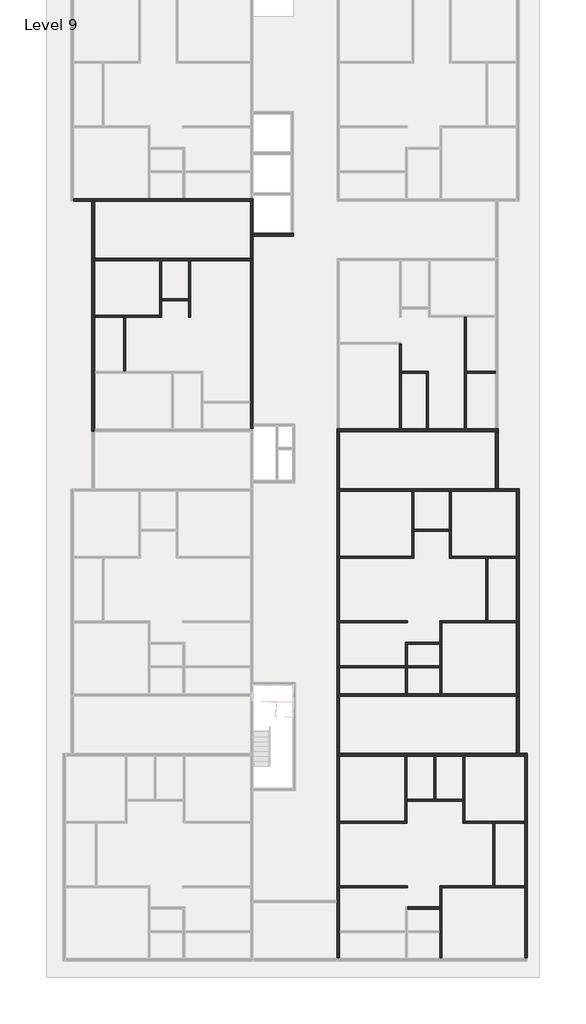
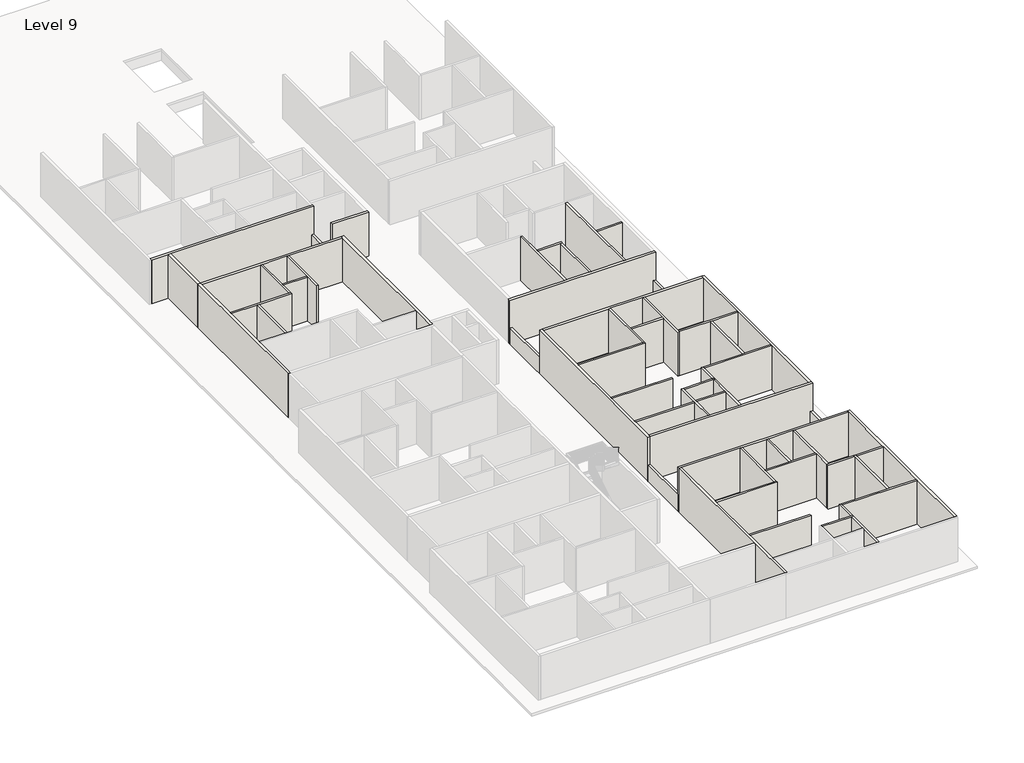
# One storey, part 2 of 8: 56 walls.
"""IFC4 building model written with IfcOpenShell, lengths in millimetres."""

from ifc_helpers import new_model, si_unit, frame, origin, place, context, project, spatial, polyline, outline, extrude, faceted_brep, element, save

model = new_model("IFC4")

# Units and contexts
model_context = context("Model", 3, world=origin())
ifc_project = project(units=[si_unit("LENGTHUNIT", "METRE", prefix="MILLI")], contexts=[model_context])

# Site, building, storey
site = spatial("IfcSite", under=ifc_project)
building = spatial("IfcBuilding", under=site)
storey = spatial("IfcBuildingStorey", under=building, Name="Level 9", Elevation=49618.6172466)

# Walls
placement = place(None, origin())
element("IfcWall", 1, ObjectType="4.5\"", at=placement, inside=storey, context=model_context, shape_type="Brep", body=[
    faceted_brep([(-12531.5544854, 2100.0216096, 49618.6172466), (-10907.2415084, 2100.0216096, 49618.6172466), (-10792.9415084, 2100.0216096, 49618.6172466), (-8759.6544854, 2100.0216096, 49618.6172466), (-8759.6544854, 2100.0216096, 52666.6172466), (-10792.9415084, 2100.0216096, 52666.6172466), (-10907.2415084, 2100.0216096, 52666.6172466), (-12531.5544854, 2100.0216096, 52666.6172466), (-12531.5544854, 2214.3216096, 49618.6172466), (-12531.5544854, 2214.3216096, 52666.6172466), (-8873.9544854, 2214.3216096, 52666.6172466), (-8759.6544854, 2214.3216096, 52666.6172466), (-8759.6544854, 2214.3216096, 49618.6172466), (-8873.9544854, 2214.3216096, 49618.6172466)], [[[0, 1, 2, 3, 4, 5, 6, 7]], [[8, 9, 10, 11, 12, 13]], [[3, 2, 1, 0, 8, 13, 12]], [[0, 7, 9, 8]], [[4, 3, 12, 11]], [[7, 6, 5, 4, 11, 10, 9]]]),
])
element("IfcWall", 2, ObjectType="4.5\"", at=placement, inside=storey, context=model_context, shape_type="Brep", body=[
    faceted_brep([(-8759.6544854, 2214.3216096, 49618.6172466), (-8759.6544854, 3014.4216096, 49618.6172466), (-8759.6544854, 3128.7216096, 49618.6172466), (-8759.6544854, 5264.2743917, 49618.6172466), (-8759.6544854, 5264.2743917, 52666.6172466), (-8759.6544854, 3128.7216096, 52666.6172466), (-8759.6544854, 3014.4216096, 52666.6172466), (-8759.6544854, 2214.3216096, 52666.6172466), (-8873.9544854, 2214.3216096, 49618.6172466), (-8873.9544854, 2214.3216096, 52666.6172466), (-8873.9544854, 5264.2743917, 52666.6172466), (-8873.9544854, 5264.2743917, 49618.6172466)], [[[0, 1, 2, 3, 4, 5, 6, 7]], [[8, 9, 10, 11]], [[3, 2, 1, 0, 8, 11]], [[0, 7, 9, 8]], [[4, 3, 11, 10]], [[7, 6, 5, 4, 10, 9]]]),
])
element("IfcWall", 3, ObjectType="4.5\"", at=placement, inside=storey, context=model_context, shape_type="Brep", body=[
    faceted_brep([(-7235.6544854, 5264.2743917, 49618.6172466), (-7235.6544854, 3128.7216096, 49618.6172466), (-7235.6544854, 3014.4216096, 49618.6172466), (-7235.6544854, 2100.0216096, 49618.6172466), (-7235.6544854, 2100.0216096, 52666.6172466), (-7235.6544854, 3014.4216096, 52666.6172466), (-7235.6544854, 3128.7216096, 52666.6172466), (-7235.6544854, 5264.2743917, 52666.6172466), (-7121.3544854, 5264.2743917, 49618.6172466), (-7121.3544854, 5264.2743917, 52666.6172466), (-7121.3544854, 2100.0216096, 52666.6172466), (-7121.3544854, 2100.0216096, 49618.6172466)], [[[0, 1, 2, 3, 4, 5, 6, 7]], [[8, 9, 10, 11]], [[3, 2, 1, 0, 8, 11]], [[4, 3, 11, 10]], [[0, 7, 9, 8]], [[7, 6, 5, 4, 10, 9]]]),
])
element("IfcWall", 4, ObjectType="4.5\"", at=placement, inside=storey, context=model_context, shape_type="SweptSolid", body=[
    extrude(outline(polyline([(-7235.6544854, 3014.4216096), (-8759.6544854, 3014.4216096), (-8759.6544854, 3128.7216096), (-7235.6544854, 3128.7216096), (-7235.6544854, 3014.4216096)])), frame((0.0, 0.0, 49618.6172466), z_axis=(0.0, 0.0, 1.0), x_axis=(1.0, 0.0, 0.0)), (0.0, 0.0, 1.0), 3048.0),
])
element("IfcWall", 5, ObjectType="4.5\"", at=placement, inside=storey, context=model_context, shape_type="SweptSolid", body=[
    extrude(outline(polyline([(-10907.2415084, -947.4344126), (-10907.2415084, 2100.0216096), (-10792.9415084, 2100.0216096), (-10792.9415084, -947.4344126), (-10907.2415084, -947.4344126)])), frame((0.0, 0.0, 49618.6172466), z_axis=(0.0, 0.0, 1.0), x_axis=(1.0, 0.0, 0.0)), (0.0, 0.0, 1.0), 3048.0),
])
element("IfcWall", 6, ObjectType="4.5\"", at=placement, inside=storey, context=model_context, shape_type="Brep", body=[
    faceted_brep([(5056.6584916, -31173.4344126, 49618.6172466), (6885.4584916, -31173.4344126, 49618.6172466), (6999.7584916, -31173.4344126, 49618.6172466), (6999.7584916, -31173.4344126, 52666.6172466), (6885.4584916, -31173.4344126, 52666.6172466), (5056.6584916, -31173.4344126, 52666.6172466), (5056.6584916, -31059.1344126, 49618.6172466), (5056.6584916, -31059.1344126, 52666.6172466), (6885.4584916, -31059.1344126, 52666.6172466), (6999.7584916, -31059.1344126, 52666.6172466), (6999.7584916, -31059.1344126, 49618.6172466), (6885.4584916, -31059.1344126, 49618.6172466)], [[[0, 1, 2, 3, 4, 5]], [[6, 7, 8, 9, 10, 11]], [[2, 1, 0, 6, 11, 10]], [[0, 5, 7, 6]], [[3, 2, 10, 9]], [[5, 4, 3, 9, 8, 7]]]),
])
element("IfcWall", 7, ObjectType="4.5\"", at=placement, inside=storey, context=model_context, shape_type="Brep", body=[
    faceted_brep([(6885.4584916, -31173.4344126, 49618.6172466), (6885.4584916, -32392.6344126, 49618.6172466), (6885.4584916, -32506.9344126, 49618.6172466), (6885.4584916, -33954.7344126, 49618.6172466), (6885.4584916, -33954.7344126, 52666.6172466), (6885.4584916, -32506.9344126, 52666.6172466), (6885.4584916, -32392.6344126, 52666.6172466), (6885.4584916, -31173.4344126, 52666.6172466), (6999.7584916, -31173.4344126, 49618.6172466), (6999.7584916, -31173.4344126, 52666.6172466), (6999.7584916, -33954.7344126, 52666.6172466), (6999.7584916, -33954.7344126, 49618.6172466)], [[[0, 1, 2, 3, 4, 5, 6, 7]], [[8, 9, 10, 11]], [[3, 2, 1, 0, 8, 11]], [[0, 7, 9, 8]], [[4, 3, 11, 10]], [[7, 6, 5, 4, 10, 9]]]),
])
element("IfcWall", 8, ObjectType="4.5\"", at=placement, inside=storey, context=model_context, shape_type="Brep", body=[
    faceted_brep([(6999.7584916, -31059.1344126, 49618.6172466), (6999.7584916, -29966.9344126, 49618.6172466), (6999.7584916, -29852.6344126, 49618.6172466), (6999.7584916, -29852.6344126, 52666.6172466), (6999.7584916, -29966.9344126, 52666.6172466), (6999.7584916, -31059.1344126, 52666.6172466), (6885.4584916, -31059.1344126, 49618.6172466), (6885.4584916, -31059.1344126, 52666.6172466), (6885.4584916, -29852.6344126, 52666.6172466), (6885.4584916, -29852.6344126, 49618.6172466)], [[[0, 1, 2, 3, 4, 5]], [[6, 7, 8, 9]], [[2, 1, 0, 6, 9]], [[0, 5, 7, 6]], [[3, 2, 9, 8]], [[5, 4, 3, 8, 7]]]),
])
element("IfcWall", 9, ObjectType="4.5\"", at=placement, inside=storey, context=model_context, shape_type="Brep", body=[
    faceted_brep([(6999.7584916, -29966.9344126, 49618.6172466), (11660.6584916, -29966.9344126, 49618.6172466), (11660.6584916, -29966.9344126, 52666.6172466), (6999.7584916, -29966.9344126, 52666.6172466), (6999.7584916, -29852.6344126, 49618.6172466), (6999.7584916, -29852.6344126, 52666.6172466), (9869.9584916, -29852.6344126, 52666.6172466), (9984.2584916, -29852.6344126, 52666.6172466), (11660.6584916, -29852.6344126, 52666.6172466), (11660.6584916, -29852.6344126, 49618.6172466), (9984.2584916, -29852.6344126, 49618.6172466), (9869.9584916, -29852.6344126, 49618.6172466)], [[[0, 1, 2, 3]], [[4, 5, 6, 7, 8, 9, 10, 11]], [[1, 0, 4, 11, 10, 9]], [[0, 3, 5, 4]], [[2, 1, 9, 8]], [[3, 2, 8, 7, 6, 5]]]),
])
element("IfcWall", 10, ObjectType="4.5\"", at=placement, inside=storey, context=model_context, shape_type="SweptSolid", body=[
    extrude(outline(polyline([(5056.6584916, -29966.9344126), (1259.3584916, -29966.9344126), (1259.3584916, -29852.6344126), (5056.6584916, -29852.6344126), (5056.6584916, -29966.9344126)])), frame((0.0, 0.0, 49618.6172466), z_axis=(0.0, 0.0, 1.0), x_axis=(1.0, 0.0, 0.0)), (0.0, 0.0, 1.0), 3048.0),
])
element("IfcWall", 11, ObjectType="4.5\"", at=placement, inside=storey, context=model_context, shape_type="Brep", body=[
    faceted_brep([(1259.3584916, -26347.4344126, 49618.6172466), (5031.2584916, -26347.4344126, 49618.6172466), (5031.2584916, -26347.4344126, 52666.6172466), (1259.3584916, -26347.4344126, 52666.6172466), (1259.3584916, -26233.1344126, 49618.6172466), (1259.3584916, -26233.1344126, 52666.6172466), (4916.9584916, -26233.1344126, 52666.6172466), (5031.2584916, -26233.1344126, 52666.6172466), (5031.2584916, -26233.1344126, 49618.6172466), (4916.9584916, -26233.1344126, 49618.6172466)], [[[0, 1, 2, 3]], [[4, 5, 6, 7, 8, 9]], [[1, 0, 4, 9, 8]], [[0, 3, 5, 4]], [[2, 1, 8, 7]], [[3, 2, 7, 6, 5]]]),
])
element("IfcWall", 12, ObjectType="4.5\"", at=placement, inside=storey, context=model_context, shape_type="Brep", body=[
    faceted_brep([(5031.2584916, -26233.1344126, 49618.6172466), (5031.2584916, -25128.2344126, 49618.6172466), (5031.2584916, -25013.9344126, 49618.6172466), (5031.2584916, -22575.5344126, 49618.6172466), (5031.2584916, -22575.5344126, 52666.6172466), (5031.2584916, -25013.9344126, 52666.6172466), (5031.2584916, -25128.2344126, 52666.6172466), (5031.2584916, -26233.1344126, 52666.6172466), (4916.9584916, -26233.1344126, 49618.6172466), (4916.9584916, -26233.1344126, 52666.6172466), (4916.9584916, -22575.5344126, 52666.6172466), (4916.9584916, -22575.5344126, 49618.6172466)], [[[0, 1, 2, 3, 4, 5, 6, 7]], [[8, 9, 10, 11]], [[3, 2, 1, 0, 8, 11]], [[0, 7, 9, 8]], [[4, 3, 11, 10]], [[7, 6, 5, 4, 10, 9]]]),
])
element("IfcWall", 13, ObjectType="4.5\"", at=placement, inside=storey, context=model_context, shape_type="Brep", body=[
    faceted_brep([(9984.2584916, -29852.6344126, 49618.6172466), (9984.2584916, -26347.4344126, 49618.6172466), (9984.2584916, -26233.1344126, 49618.6172466), (9984.2584916, -26233.1344126, 52666.6172466), (9984.2584916, -26347.4344126, 52666.6172466), (9984.2584916, -29852.6344126, 52666.6172466), (9869.9584916, -29852.6344126, 49618.6172466), (9869.9584916, -29852.6344126, 52666.6172466), (9869.9584916, -26347.4344126, 52666.6172466), (9869.9584916, -26233.1344126, 52666.6172466), (9869.9584916, -26233.1344126, 49618.6172466), (9869.9584916, -26347.4344126, 49618.6172466)], [[[0, 1, 2, 3, 4, 5]], [[6, 7, 8, 9, 10, 11]], [[2, 1, 0, 6, 11, 10]], [[0, 5, 7, 6]], [[3, 2, 10, 9]], [[5, 4, 3, 9, 8, 7]]]),
])
element("IfcWall", 14, ObjectType="4.5\"", at=placement, inside=storey, context=model_context, shape_type="SweptSolid", body=[
    extrude(outline(polyline([(11660.6584916, -26347.4344126), (9984.2584916, -26347.4344126), (9984.2584916, -26233.1344126), (11660.6584916, -26233.1344126), (11660.6584916, -26347.4344126)])), frame((0.0, 0.0, 49618.6172466), z_axis=(0.0, 0.0, 1.0), x_axis=(1.0, 0.0, 0.0)), (0.0, 0.0, 1.0), 3048.0),
])
element("IfcWall", 15, ObjectType="4.5\"", at=placement, inside=storey, context=model_context, shape_type="Brep", body=[
    faceted_brep([(9869.9584916, -26233.1344126, 49618.6172466), (8307.8584916, -26233.1344126, 49618.6172466), (8193.5584916, -26233.1344126, 49618.6172466), (8193.5584916, -26233.1344126, 52666.6172466), (8307.8584916, -26233.1344126, 52666.6172466), (9869.9584916, -26233.1344126, 52666.6172466), (9869.9584916, -26347.4344126, 49618.6172466), (9869.9584916, -26347.4344126, 52666.6172466), (8193.5584916, -26347.4344126, 52666.6172466), (8193.5584916, -26347.4344126, 49618.6172466)], [[[0, 1, 2, 3, 4, 5]], [[6, 7, 8, 9]], [[2, 1, 0, 6, 9]], [[0, 5, 7, 6]], [[3, 2, 9, 8]], [[5, 4, 3, 8, 7]]]),
])
element("IfcWall", 16, ObjectType="4.5\"", at=placement, inside=storey, context=model_context, shape_type="Brep", body=[
    faceted_brep([(8307.8584916, -26233.1344126, 49618.6172466), (8307.8584916, -22575.5344126, 49618.6172466), (8307.8584916, -22575.5344126, 52666.6172466), (8307.8584916, -26233.1344126, 52666.6172466), (8193.5584916, -26233.1344126, 49618.6172466), (8193.5584916, -26233.1344126, 52666.6172466), (8193.5584916, -25128.2344126, 52666.6172466), (8193.5584916, -25013.9344126, 52666.6172466), (8193.5584916, -22575.5344126, 52666.6172466), (8193.5584916, -22575.5344126, 49618.6172466), (8193.5584916, -25013.9344126, 49618.6172466), (8193.5584916, -25128.2344126, 49618.6172466)], [[[0, 1, 2, 3]], [[4, 5, 6, 7, 8, 9, 10, 11]], [[1, 0, 4, 11, 10, 9]], [[0, 3, 5, 4]], [[2, 1, 9, 8]], [[3, 2, 8, 7, 6, 5]]]),
])
element("IfcWall", 17, ObjectType="4.5\"", at=placement, inside=storey, context=model_context, shape_type="Brep", body=[
    faceted_brep([(5031.2584916, -25128.2344126, 49618.6172466), (8193.5584916, -25128.2344126, 49618.6172466), (8193.5584916, -25128.2344126, 52666.6172466), (5031.2584916, -25128.2344126, 52666.6172466), (5031.2584916, -25013.9344126, 49618.6172466), (5031.2584916, -25013.9344126, 52666.6172466), (6555.2584916, -25013.9344126, 52666.6172466), (6669.5584916, -25013.9344126, 52666.6172466), (8193.5584916, -25013.9344126, 52666.6172466), (8193.5584916, -25013.9344126, 49618.6172466), (6669.5584916, -25013.9344126, 49618.6172466), (6555.2584916, -25013.9344126, 49618.6172466)], [[[0, 1, 2, 3]], [[4, 5, 6, 7, 8, 9, 10, 11]], [[1, 0, 4, 11, 10, 9]], [[0, 3, 5, 4]], [[2, 1, 9, 8]], [[3, 2, 8, 7, 6, 5]]]),
])
element("IfcWall", 18, ObjectType="4.5\"", at=placement, inside=storey, context=model_context, shape_type="SweptSolid", body=[
    extrude(outline(polyline([(6555.2584916, -25013.9344126), (6555.2584916, -22575.5344126), (6669.5584916, -22575.5344126), (6669.5584916, -25013.9344126), (6555.2584916, -25013.9344126)])), frame((0.0, 0.0, 49618.6172466), z_axis=(0.0, 0.0, 1.0), x_axis=(1.0, 0.0, 0.0)), (0.0, 0.0, 1.0), 3048.0),
])
element("IfcWall", 19, ObjectType="4.5\"", at=placement, inside=storey, context=model_context, shape_type="SweptSolid", body=[
    extrude(outline(polyline([(4942.3584916, -17622.5344126), (1259.3584916, -17622.5344126), (1259.3584916, -17508.2344126), (4942.3584916, -17508.2344126), (4942.3584916, -17622.5344126)])), frame((0.0, 0.0, 49618.6172466), z_axis=(0.0, 0.0, 1.0), x_axis=(1.0, 0.0, 0.0)), (0.0, 0.0, 1.0), 3048.0),
])
element("IfcWall", 20, ObjectType="4.5\"", at=placement, inside=storey, context=model_context, shape_type="Brep", body=[
    faceted_brep([(4942.3584916, -16174.7344126, 49618.6172466), (4942.3584916, -17508.2344126, 49618.6172466), (4942.3584916, -17622.5344126, 49618.6172466), (4942.3584916, -19070.3344126, 49618.6172466), (4942.3584916, -19070.3344126, 52666.6172466), (4942.3584916, -17622.5344126, 52666.6172466), (4942.3584916, -17508.2344126, 52666.6172466), (4942.3584916, -16174.7344126, 52666.6172466), (5056.6584916, -16174.7344126, 49618.6172466), (5056.6584916, -16174.7344126, 52666.6172466), (5056.6584916, -16289.0344126, 52666.6172466), (5056.6584916, -17508.2344126, 52666.6172466), (5056.6584916, -17622.5344126, 52666.6172466), (5056.6584916, -19070.3344126, 52666.6172466), (5056.6584916, -19070.3344126, 49618.6172466), (5056.6584916, -17622.5344126, 49618.6172466), (5056.6584916, -17508.2344126, 49618.6172466), (5056.6584916, -16289.0344126, 49618.6172466)], [[[0, 1, 2, 3, 4, 5, 6, 7]], [[8, 9, 10, 11, 12, 13, 14, 15, 16, 17]], [[3, 2, 1, 0, 8, 17, 16, 15, 14]], [[4, 3, 14, 13]], [[0, 7, 9, 8]], [[7, 6, 5, 4, 13, 12, 11, 10, 9]]]),
])
element("IfcWall", 21, ObjectType="4.5\"", at=placement, inside=storey, context=model_context, shape_type="Brep", body=[
    faceted_brep([(5056.6584916, -16289.0344126, 49618.6172466), (6885.4584916, -16289.0344126, 49618.6172466), (6999.7584916, -16289.0344126, 49618.6172466), (6999.7584916, -16289.0344126, 52666.6172466), (6885.4584916, -16289.0344126, 52666.6172466), (5056.6584916, -16289.0344126, 52666.6172466), (5056.6584916, -16174.7344126, 49618.6172466), (5056.6584916, -16174.7344126, 52666.6172466), (6885.4584916, -16174.7344126, 52666.6172466), (6999.7584916, -16174.7344126, 52666.6172466), (6999.7584916, -16174.7344126, 49618.6172466), (6885.4584916, -16174.7344126, 49618.6172466)], [[[0, 1, 2, 3, 4, 5]], [[6, 7, 8, 9, 10, 11]], [[2, 1, 0, 6, 11, 10]], [[0, 5, 7, 6]], [[3, 2, 10, 9]], [[5, 4, 3, 9, 8, 7]]]),
])
element("IfcWall", 22, ObjectType="4.5\"", at=placement, inside=storey, context=model_context, shape_type="Brep", body=[
    faceted_brep([(6885.4584916, -16289.0344126, 49618.6172466), (6885.4584916, -17508.2344126, 49618.6172466), (6885.4584916, -17622.5344126, 49618.6172466), (6885.4584916, -19070.3344126, 49618.6172466), (6885.4584916, -19070.3344126, 52666.6172466), (6885.4584916, -17622.5344126, 52666.6172466), (6885.4584916, -17508.2344126, 52666.6172466), (6885.4584916, -16289.0344126, 52666.6172466), (6999.7584916, -16289.0344126, 49618.6172466), (6999.7584916, -16289.0344126, 52666.6172466), (6999.7584916, -19070.3344126, 52666.6172466), (6999.7584916, -19070.3344126, 49618.6172466)], [[[0, 1, 2, 3, 4, 5, 6, 7]], [[8, 9, 10, 11]], [[3, 2, 1, 0, 8, 11]], [[0, 7, 9, 8]], [[4, 3, 11, 10]], [[7, 6, 5, 4, 10, 9]]]),
])
element("IfcWall", 23, ObjectType="4.5\"", at=placement, inside=storey, context=model_context, shape_type="SweptSolid", body=[
    extrude(outline(polyline([(6885.4584916, -17622.5344126), (5056.6584916, -17622.5344126), (5056.6584916, -17508.2344126), (6885.4584916, -17508.2344126), (6885.4584916, -17622.5344126)])), frame((0.0, 0.0, 49618.6172466), z_axis=(0.0, 0.0, 1.0), x_axis=(1.0, 0.0, 0.0)), (0.0, 0.0, 1.0), 3048.0),
])
element("IfcWall", 24, ObjectType="4.5\"", at=placement, inside=storey, context=model_context, shape_type="Brep", body=[
    faceted_brep([(6999.7584916, -16174.7344126, 49618.6172466), (6999.7584916, -15082.5344126, 49618.6172466), (6999.7584916, -14968.2344126, 49618.6172466), (6999.7584916, -14968.2344126, 52666.6172466), (6999.7584916, -15082.5344126, 52666.6172466), (6999.7584916, -16174.7344126, 52666.6172466), (6885.4584916, -16174.7344126, 49618.6172466), (6885.4584916, -16174.7344126, 52666.6172466), (6885.4584916, -14968.2344126, 52666.6172466), (6885.4584916, -14968.2344126, 49618.6172466)], [[[0, 1, 2, 3, 4, 5]], [[6, 7, 8, 9]], [[2, 1, 0, 6, 9]], [[0, 5, 7, 6]], [[3, 2, 9, 8]], [[5, 4, 3, 8, 7]]]),
])
element("IfcWall", 25, ObjectType="4.5\"", at=placement, inside=storey, context=model_context, shape_type="Brep", body=[
    faceted_brep([(6999.7584916, -15082.5344126, 49618.6172466), (11208.5214687, -15082.5344126, 49618.6172466), (11208.5214687, -15082.5344126, 52666.6172466), (6999.7584916, -15082.5344126, 52666.6172466), (6999.7584916, -14968.2344126, 49618.6172466), (6999.7584916, -14968.2344126, 52666.6172466), (9469.9084916, -14968.2344126, 52666.6172466), (9584.2084916, -14968.2344126, 52666.6172466), (11208.5214687, -14968.2344126, 52666.6172466), (11208.5214687, -14968.2344126, 49618.6172466), (9584.2084916, -14968.2344126, 49618.6172466), (9469.9084916, -14968.2344126, 49618.6172466)], [[[0, 1, 2, 3]], [[4, 5, 6, 7, 8, 9, 10, 11]], [[1, 0, 4, 11, 10, 9]], [[0, 3, 5, 4]], [[2, 1, 9, 8]], [[3, 2, 8, 7, 6, 5]]]),
])
element("IfcWall", 26, ObjectType="4.5\"", at=placement, inside=storey, context=model_context, shape_type="SweptSolid", body=[
    extrude(outline(polyline([(5056.6584916, -15082.5344126), (1259.3584916, -15082.5344126), (1259.3584916, -14968.2344126), (5056.6584916, -14968.2344126), (5056.6584916, -15082.5344126)])), frame((0.0, 0.0, 49618.6172466), z_axis=(0.0, 0.0, 1.0), x_axis=(1.0, 0.0, 0.0)), (0.0, 0.0, 1.0), 3048.0),
])
element("IfcWall", 27, ObjectType="4.5\"", at=placement, inside=storey, context=model_context, shape_type="Brep", body=[
    faceted_brep([(1259.3584916, -11463.0344126, 49618.6172466), (5430.0214687, -11463.0344126, 49618.6172466), (5430.0214687, -11463.0344126, 52666.6172466), (1259.3584916, -11463.0344126, 52666.6172466), (1259.3584916, -11348.7344126, 49618.6172466), (1259.3584916, -11348.7344126, 52666.6172466), (5315.7214687, -11348.7344126, 52666.6172466), (5430.0214687, -11348.7344126, 52666.6172466), (5430.0214687, -11348.7344126, 49618.6172466), (5315.7214687, -11348.7344126, 49618.6172466)], [[[0, 1, 2, 3]], [[4, 5, 6, 7, 8, 9]], [[1, 0, 4, 9, 8]], [[0, 3, 5, 4]], [[2, 1, 8, 7]], [[3, 2, 7, 6, 5]]]),
])
element("IfcWall", 28, ObjectType="4.5\"", at=placement, inside=storey, context=model_context, shape_type="Brep", body=[
    faceted_brep([(5430.0214687, -11348.7344126, 49618.6172466), (5430.0214687, -9939.0344126, 49618.6172466), (5430.0214687, -9824.7344126, 49618.6172466), (5430.0214687, -7691.1344126, 49618.6172466), (5430.0214687, -7691.1344126, 52666.6172466), (5430.0214687, -9824.7344126, 52666.6172466), (5430.0214687, -9939.0344126, 52666.6172466), (5430.0214687, -11348.7344126, 52666.6172466), (5315.7214687, -11348.7344126, 49618.6172466), (5315.7214687, -11348.7344126, 52666.6172466), (5315.7214687, -7691.1344126, 52666.6172466), (5315.7214687, -7691.1344126, 49618.6172466)], [[[0, 1, 2, 3, 4, 5, 6, 7]], [[8, 9, 10, 11]], [[3, 2, 1, 0, 8, 11]], [[0, 7, 9, 8]], [[4, 3, 11, 10]], [[7, 6, 5, 4, 10, 9]]]),
])
element("IfcWall", 29, ObjectType="4.5\"", at=placement, inside=storey, context=model_context, shape_type="SweptSolid", body=[
    extrude(outline(polyline([(7436.6214687, -9939.0344126), (5430.0214687, -9939.0344126), (5430.0214687, -9824.7344126), (7436.6214687, -9824.7344126), (7436.6214687, -9939.0344126)])), frame((0.0, 0.0, 49618.6172466), z_axis=(0.0, 0.0, 1.0), x_axis=(1.0, 0.0, 0.0)), (0.0, 0.0, 1.0), 3048.0),
])
element("IfcWall", 30, ObjectType="4.5\"", at=placement, inside=storey, context=model_context, shape_type="Brep", body=[
    faceted_brep([(7436.6214687, -7691.1344126, 49618.6172466), (7436.6214687, -9824.7344126, 49618.6172466), (7436.6214687, -9939.0344126, 49618.6172466), (7436.6214687, -11463.0344126, 49618.6172466), (7436.6214687, -11463.0344126, 52666.6172466), (7436.6214687, -9939.0344126, 52666.6172466), (7436.6214687, -9824.7344126, 52666.6172466), (7436.6214687, -7691.1344126, 52666.6172466), (7550.9214687, -7691.1344126, 49618.6172466), (7550.9214687, -7691.1344126, 52666.6172466), (7550.9214687, -11348.7344126, 52666.6172466), (7550.9214687, -11463.0344126, 52666.6172466), (7550.9214687, -11463.0344126, 49618.6172466), (7550.9214687, -11348.7344126, 49618.6172466)], [[[0, 1, 2, 3, 4, 5, 6, 7]], [[8, 9, 10, 11, 12, 13]], [[3, 2, 1, 0, 8, 13, 12]], [[0, 7, 9, 8]], [[4, 3, 12, 11]], [[7, 6, 5, 4, 11, 10, 9]]]),
])
element("IfcWall", 31, ObjectType="4.5\"", at=placement, inside=storey, context=model_context, shape_type="Brep", body=[
    faceted_brep([(7550.9214687, -11463.0344126, 49618.6172466), (9469.9084916, -11463.0344126, 49618.6172466), (9584.2084916, -11463.0344126, 49618.6172466), (11208.5214687, -11463.0344126, 49618.6172466), (11208.5214687, -11463.0344126, 52666.6172466), (9584.2084916, -11463.0344126, 52666.6172466), (9469.9084916, -11463.0344126, 52666.6172466), (7550.9214687, -11463.0344126, 52666.6172466), (7550.9214687, -11348.7344126, 49618.6172466), (7550.9214687, -11348.7344126, 52666.6172466), (11208.5214687, -11348.7344126, 52666.6172466), (11208.5214687, -11348.7344126, 49618.6172466)], [[[0, 1, 2, 3, 4, 5, 6, 7]], [[8, 9, 10, 11]], [[3, 2, 1, 0, 8, 11]], [[0, 7, 9, 8]], [[4, 3, 11, 10]], [[7, 6, 5, 4, 10, 9]]]),
])
element("IfcWall", 32, ObjectType="4.5\"", at=placement, inside=storey, context=model_context, shape_type="SweptSolid", body=[
    extrude(outline(polyline([(9469.9084916, -14968.2344126), (9469.9084916, -11463.0344126), (9584.2084916, -11463.0344126), (9584.2084916, -14968.2344126), (9469.9084916, -14968.2344126)])), frame((0.0, 0.0, 49618.6172466), z_axis=(0.0, 0.0, 1.0), x_axis=(1.0, 0.0, 0.0)), (0.0, 0.0, 1.0), 3048.0),
])
element("IfcWall", 33, ObjectType="4.5\"", at=placement, inside=storey, context=model_context, shape_type="Brep", body=[
    faceted_brep([(4610.8714687, 572.7745083, 49618.6172466), (4610.8714687, -4185.9344126, 49618.6172466), (4610.8714687, -4185.9344126, 52666.6172466), (4610.8714687, 572.7745083, 52666.6172466), (4725.1714687, 572.7745083, 49618.6172466), (4725.1714687, 572.7745083, 52666.6172466), (4725.1714687, -947.4344126, 52666.6172466), (4725.1714687, -1061.7344126, 52666.6172466), (4725.1714687, -4185.9344126, 52666.6172466), (4725.1714687, -4185.9344126, 49618.6172466), (4725.1714687, -1061.7344126, 49618.6172466), (4725.1714687, -947.4344126, 49618.6172466)], [[[0, 1, 2, 3]], [[4, 5, 6, 7, 8, 9, 10, 11]], [[1, 0, 4, 11, 10, 9]], [[0, 3, 5, 4]], [[2, 1, 9, 8]], [[3, 2, 8, 7, 6, 5]]]),
])
element("IfcWall", 34, ObjectType="4.5\"", at=placement, inside=storey, context=model_context, shape_type="Brep", body=[
    faceted_brep([(4725.1714687, -1061.7344126, 49618.6172466), (6134.8714687, -1061.7344126, 49618.6172466), (6249.1714687, -1061.7344126, 49618.6172466), (6249.1714687, -1061.7344126, 52666.6172466), (6134.8714687, -1061.7344126, 52666.6172466), (4725.1714687, -1061.7344126, 52666.6172466), (4725.1714687, -947.4344126, 49618.6172466), (4725.1714687, -947.4344126, 52666.6172466), (6249.1714687, -947.4344126, 52666.6172466), (6249.1714687, -947.4344126, 49618.6172466)], [[[0, 1, 2, 3, 4, 5]], [[6, 7, 8, 9]], [[2, 1, 0, 6, 9]], [[0, 5, 7, 6]], [[3, 2, 9, 8]], [[5, 4, 3, 8, 7]]]),
])
element("IfcWall", 35, ObjectType="4.5\"", at=placement, inside=storey, context=model_context, shape_type="SweptSolid", body=[
    extrude(outline(polyline([(6134.8714687, -4185.9344126), (6134.8714687, -1061.7344126), (6249.1714687, -1061.7344126), (6249.1714687, -4185.9344126), (6134.8714687, -4185.9344126)])), frame((0.0, 0.0, 49618.6172466), z_axis=(0.0, 0.0, 1.0), x_axis=(1.0, 0.0, 0.0)), (0.0, 0.0, 1.0), 3048.0),
])
element("IfcWall", 36, ObjectType="4.5\"", at=placement, inside=storey, context=model_context, shape_type="Brep", body=[
    faceted_brep([(8396.7584916, -4185.9344126, 49618.6172466), (8396.7584916, -1061.7344126, 49618.6172466), (8396.7584916, -947.4344126, 49618.6172466), (8396.7584916, 2100.0216096, 49618.6172466), (8396.7584916, 2100.0216096, 52666.6172466), (8396.7584916, -947.4344126, 52666.6172466), (8396.7584916, -1061.7344126, 52666.6172466), (8396.7584916, -4185.9344126, 52666.6172466), (8282.4584916, -4185.9344126, 49618.6172466), (8282.4584916, -4185.9344126, 52666.6172466), (8282.4584916, 2100.0216096, 52666.6172466), (8282.4584916, 2100.0216096, 49618.6172466)], [[[0, 1, 2, 3, 4, 5, 6, 7]], [[8, 9, 10, 11]], [[3, 2, 1, 0, 8, 11]], [[0, 7, 9, 8]], [[4, 3, 11, 10]], [[7, 6, 5, 4, 10, 9]]]),
])
element("IfcWall", 37, ObjectType="4.5\"", at=placement, inside=storey, context=model_context, shape_type="SweptSolid", body=[
    extrude(outline(polyline([(8396.7584916, -947.4344126), (10021.0714687, -947.4344126), (10021.0714687, -1061.7344126), (8396.7584916, -1061.7344126), (8396.7584916, -947.4344126)])), frame((0.0, 0.0, 49618.6172466), z_axis=(0.0, 0.0, 1.0), x_axis=(1.0, 0.0, 0.0)), (0.0, 0.0, 1.0), 3048.0),
])
element("IfcWall", 38, ObjectType="6\"", at=placement, inside=storey, context=model_context, shape_type="Brep", body=[
    faceted_brep([(-13719.0044854, 8615.1216096, 49618.6172466), (-12683.9544854, 8615.1216096, 49618.6172466), (-12531.5544854, 8615.1216096, 49618.6172466), (-3769.8415084, 8615.1216096, 49618.6172466), (-3617.4415084, 8615.1216096, 49618.6172466), (-3617.4415084, 8615.1216096, 50837.8172466), (-3617.4415084, 8615.1216096, 52666.6172466), (-12531.5544854, 8615.1216096, 52666.6172466), (-12683.9544854, 8615.1216096, 52666.6172466), (-13719.0044854, 8615.1216096, 52666.6172466), (-13719.0044854, 8767.5216096, 49618.6172466), (-13719.0044854, 8767.5216096, 52666.6172466), (-9510.2415084, 8767.5216096, 52666.6172466), (-9395.9415084, 8767.5216096, 52666.6172466), (-7567.1415084, 8767.5216096, 52666.6172466), (-7452.8415084, 8767.5216096, 52666.6172466), (-3769.8415084, 8767.5216096, 52666.6172466), (-3617.4415084, 8767.5216096, 52666.6172466), (-3617.4415084, 8767.5216096, 49618.6172466), (-3769.8415084, 8767.5216096, 49618.6172466), (-7452.8415084, 8767.5216096, 49618.6172466), (-7567.1415084, 8767.5216096, 49618.6172466), (-9395.9415084, 8767.5216096, 49618.6172466), (-9510.2415084, 8767.5216096, 49618.6172466)], [[[0, 1, 2, 3, 4, 5, 6, 7, 8, 9]], [[10, 11, 12, 13, 14, 15, 16, 17, 18, 19, 20, 21, 22, 23]], [[4, 3, 2, 1, 0, 10, 23, 22, 21, 20, 19, 18]], [[0, 9, 11, 10]], [[4, 18, 17, 6, 5]], [[9, 8, 7, 6, 17, 16, 15, 14, 13, 12, 11]]]),
])
element("IfcWall", 39, ObjectType="6\"", at=placement, inside=storey, context=model_context, shape_type="Brep", body=[
    faceted_brep([(-12683.9544854, 5416.6743917, 49618.6172466), (-12683.9544854, -4338.3344126, 49618.6172466), (-12683.9544854, -4338.3344126, 52666.6172466), (-12683.9544854, 5416.6743917, 52666.6172466), (-12531.5544854, 5416.6743917, 49618.6172466), (-12531.5544854, 5416.6743917, 52666.6172466), (-12531.5544854, 5264.2743917, 52666.6172466), (-12531.5544854, 2214.3216096, 52666.6172466), (-12531.5544854, 2100.0216096, 52666.6172466), (-12531.5544854, -947.4344126, 52666.6172466), (-12531.5544854, -1061.7344126, 52666.6172466), (-12531.5544854, -4185.9344126, 52666.6172466), (-12531.5544854, -4338.3344126, 52666.6172466), (-12531.5544854, -4338.3344126, 49618.6172466), (-12531.5544854, -4185.9344126, 49618.6172466), (-12531.5544854, -1061.7344126, 49618.6172466), (-12531.5544854, -947.4344126, 49618.6172466), (-12531.5544854, 2100.0216096, 49618.6172466), (-12531.5544854, 2214.3216096, 49618.6172466), (-12531.5544854, 5264.2743917, 49618.6172466)], [[[0, 1, 2, 3]], [[4, 5, 6, 7, 8, 9, 10, 11, 12, 13, 14, 15, 16, 17, 18, 19]], [[1, 0, 4, 19, 18, 17, 16, 15, 14, 13]], [[2, 1, 13, 12]], [[0, 3, 5, 4]], [[3, 2, 12, 11, 10, 9, 8, 7, 6, 5]]]),
])
element("IfcWall", 40, ObjectType="6\"", at=placement, inside=storey, context=model_context, shape_type="Brep", body=[
    faceted_brep([(-3617.4415084, -4185.9344126, 49618.6172466), (-3617.4415084, -4034.6751812, 49618.6172466), (-3617.4415084, -3882.2751812, 49618.6172466), (-3617.4415084, 5416.6743917, 49618.6172466), (-3617.4415084, 5416.6743917, 52666.6172466), (-3617.4415084, -3882.2751812, 52666.6172466), (-3617.4415084, -4034.6751812, 52666.6172466), (-3617.4415084, -4185.9344126, 52666.6172466), (-3769.8415084, -4185.9344126, 49618.6172466), (-3769.8415084, -4185.9344126, 52666.6172466), (-3769.8415084, -2738.1344126, 52666.6172466), (-3769.8415084, -2623.8344126, 52666.6172466), (-3769.8415084, 5264.2743917, 52666.6172466), (-3769.8415084, 5416.6743917, 52666.6172466), (-3769.8415084, 5416.6743917, 49618.6172466), (-3769.8415084, 5264.2743917, 49618.6172466), (-3769.8415084, -2623.8344126, 49618.6172466), (-3769.8415084, -2738.1344126, 49618.6172466)], [[[0, 1, 2, 3, 4, 5, 6, 7]], [[8, 9, 10, 11, 12, 13, 14, 15, 16, 17]], [[3, 2, 1, 0, 8, 17, 16, 15, 14]], [[0, 7, 9, 8]], [[3, 14, 13, 4]], [[7, 6, 5, 4, 13, 12, 11, 10, 9]]]),
])
element("IfcWall", 41, ObjectType="6\"", at=placement, inside=storey, context=model_context, shape_type="Brep", body=[
    faceted_brep([(-3769.8415084, 5416.6743917, 52666.6172466), (-3769.8415084, 5416.6743917, 49618.6172466), (-12531.5544854, 5416.6743917, 49618.6172466), (-12531.5544854, 5416.6743917, 52666.6172466), (-3769.8415084, 5264.2743917, 49618.6172466), (-3769.8415084, 5264.2743917, 52666.6172466), (-7121.3544854, 5264.2743917, 52666.6172466), (-7235.6544854, 5264.2743917, 52666.6172466), (-8759.6544854, 5264.2743917, 52666.6172466), (-8873.9544854, 5264.2743917, 52666.6172466), (-12531.5544854, 5264.2743917, 52666.6172466), (-12531.5544854, 5264.2743917, 49618.6172466), (-8873.9544854, 5264.2743917, 49618.6172466), (-8759.6544854, 5264.2743917, 49618.6172466), (-7235.6544854, 5264.2743917, 49618.6172466), (-7121.3544854, 5264.2743917, 49618.6172466)], [[[0, 1, 2, 3]], [[4, 5, 6, 7, 8, 9, 10, 11, 12, 13, 14, 15]], [[2, 1, 4, 15, 14, 13, 12, 11]], [[3, 2, 11, 10]], [[0, 5, 4, 1]], [[0, 3, 10, 9, 8, 7, 6, 5]]]),
])
element("IfcWall", 42, ObjectType="6\"", at=placement, inside=storey, context=model_context, shape_type="Brep", body=[
    faceted_brep([(11813.0584916, -33954.7344126, 49618.6172466), (11813.0584916, -22423.1344126, 49618.6172466), (11813.0584916, -22423.1344126, 52666.6172466), (11813.0584916, -33954.7344126, 52666.6172466), (11660.6584916, -33954.7344126, 49618.6172466), (11660.6584916, -33954.7344126, 52666.6172466), (11660.6584916, -29966.9344126, 52666.6172466), (11660.6584916, -29852.6344126, 52666.6172466), (11660.6584916, -26347.4344126, 52666.6172466), (11660.6584916, -26233.1344126, 52666.6172466), (11660.6584916, -22575.5344126, 52666.6172466), (11660.6584916, -22423.1344126, 52666.6172466), (11660.6584916, -22423.1344126, 49618.6172466), (11660.6584916, -22575.5344126, 49618.6172466), (11660.6584916, -26233.1344126, 49618.6172466), (11660.6584916, -26347.4344126, 49618.6172466), (11660.6584916, -29852.6344126, 49618.6172466), (11660.6584916, -29966.9344126, 49618.6172466)], [[[0, 1, 2, 3]], [[4, 5, 6, 7, 8, 9, 10, 11, 12, 13, 14, 15, 16, 17]], [[1, 0, 4, 17, 16, 15, 14, 13, 12]], [[0, 3, 5, 4]], [[2, 1, 12, 11]], [[3, 2, 11, 10, 9, 8, 7, 6, 5]]]),
])
element("IfcWall", 43, ObjectType="6\"", at=placement, inside=storey, context=model_context, shape_type="Brep", body=[
    faceted_brep([(11660.6584916, -22423.1344126, 49618.6172466), (11360.9214687, -22423.1344126, 49618.6172466), (11208.5214687, -22423.1344126, 49618.6172466), (1259.3584916, -22423.1344126, 49618.6172466), (1106.9584916, -22423.1344126, 49618.6172466), (1106.9584916, -22423.1344126, 50837.8172466), (1106.9584916, -22423.1344126, 52666.6172466), (11660.6584916, -22423.1344126, 52666.6172466), (11660.6584916, -22575.5344126, 49618.6172466), (11660.6584916, -22575.5344126, 52666.6172466), (8307.8584916, -22575.5344126, 52666.6172466), (8193.5584916, -22575.5344126, 52666.6172466), (6669.5584916, -22575.5344126, 52666.6172466), (6555.2584916, -22575.5344126, 52666.6172466), (5031.2584916, -22575.5344126, 52666.6172466), (4916.9584916, -22575.5344126, 52666.6172466), (1259.3584916, -22575.5344126, 52666.6172466), (1106.9584916, -22575.5344126, 52666.6172466), (1106.9584916, -22575.5344126, 49618.6172466), (1259.3584916, -22575.5344126, 49618.6172466), (4916.9584916, -22575.5344126, 49618.6172466), (5031.2584916, -22575.5344126, 49618.6172466), (6555.2584916, -22575.5344126, 49618.6172466), (6669.5584916, -22575.5344126, 49618.6172466), (8193.5584916, -22575.5344126, 49618.6172466), (8307.8584916, -22575.5344126, 49618.6172466)], [[[0, 1, 2, 3, 4, 5, 6, 7]], [[8, 9, 10, 11, 12, 13, 14, 15, 16, 17, 18, 19, 20, 21, 22, 23, 24, 25]], [[4, 3, 2, 1, 0, 8, 25, 24, 23, 22, 21, 20, 19, 18]], [[0, 7, 9, 8]], [[4, 18, 17, 6, 5]], [[7, 6, 17, 16, 15, 14, 13, 12, 11, 10, 9]]]),
])
element("IfcWall", 44, ObjectType="6\"", at=placement, inside=storey, context=model_context, shape_type="Brep", body=[
    faceted_brep([(1106.9584916, -22575.5344126, 52666.6172466), (1106.9584916, -22575.5344126, 49618.6172466), (1106.9584916, -30668.5325185, 49618.6172466), (1106.9584916, -30820.9325185, 49618.6172466), (1106.9584916, -33954.7344126, 49618.6172466), (1106.9584916, -33954.7344126, 52666.6172466), (1106.9584916, -30820.9325185, 52666.6172466), (1106.9584916, -30668.5325185, 52666.6172466), (1259.3584916, -22575.5344126, 49618.6172466), (1259.3584916, -22575.5344126, 52666.6172466), (1259.3584916, -26233.1344126, 52666.6172466), (1259.3584916, -26347.4344126, 52666.6172466), (1259.3584916, -29852.6344126, 52666.6172466), (1259.3584916, -29966.9344126, 52666.6172466), (1259.3584916, -32392.6344126, 52666.6172466), (1259.3584916, -32506.9344126, 52666.6172466), (1259.3584916, -33954.7344126, 52666.6172466), (1259.3584916, -33954.7344126, 49618.6172466), (1259.3584916, -32506.9344126, 49618.6172466), (1259.3584916, -32392.6344126, 49618.6172466), (1259.3584916, -29966.9344126, 49618.6172466), (1259.3584916, -29852.6344126, 49618.6172466), (1259.3584916, -26347.4344126, 49618.6172466), (1259.3584916, -26233.1344126, 49618.6172466)], [[[0, 1, 2, 3, 4, 5, 6, 7]], [[8, 9, 10, 11, 12, 13, 14, 15, 16, 17, 18, 19, 20, 21, 22, 23]], [[4, 3, 2, 1, 8, 23, 22, 21, 20, 19, 18, 17]], [[5, 4, 17, 16]], [[0, 9, 8, 1]], [[0, 7, 6, 5, 16, 15, 14, 13, 12, 11, 10, 9]]]),
])
element("IfcWall", 45, ObjectType="6\"", at=placement, inside=storey, context=model_context, shape_type="Brep", body=[
    faceted_brep([(1106.9584916, -7538.7344126, 52666.6172466), (1106.9584916, -7538.7344126, 49618.6172466), (1106.9584916, -19222.7344126, 49618.6172466), (1106.9584916, -19222.7344126, 52666.6172466), (1259.3584916, -7538.7344126, 49618.6172466), (1259.3584916, -7538.7344126, 52666.6172466), (1259.3584916, -7691.1344126, 52666.6172466), (1259.3584916, -11348.7344126, 52666.6172466), (1259.3584916, -11463.0344126, 52666.6172466), (1259.3584916, -14968.2344126, 52666.6172466), (1259.3584916, -15082.5344126, 52666.6172466), (1259.3584916, -17508.2344126, 52666.6172466), (1259.3584916, -17622.5344126, 52666.6172466), (1259.3584916, -19070.3344126, 52666.6172466), (1259.3584916, -19222.7344126, 52666.6172466), (1259.3584916, -19222.7344126, 49618.6172466), (1259.3584916, -19070.3344126, 49618.6172466), (1259.3584916, -17622.5344126, 49618.6172466), (1259.3584916, -17508.2344126, 49618.6172466), (1259.3584916, -15082.5344126, 49618.6172466), (1259.3584916, -14968.2344126, 49618.6172466), (1259.3584916, -11463.0344126, 49618.6172466), (1259.3584916, -11348.7344126, 49618.6172466), (1259.3584916, -7691.1344126, 49618.6172466)], [[[0, 1, 2, 3]], [[4, 5, 6, 7, 8, 9, 10, 11, 12, 13, 14, 15, 16, 17, 18, 19, 20, 21, 22, 23]], [[2, 1, 4, 23, 22, 21, 20, 19, 18, 17, 16, 15]], [[0, 5, 4, 1]], [[2, 15, 14, 3]], [[0, 3, 14, 13, 12, 11, 10, 9, 8, 7, 6, 5]]]),
])
element("IfcWall", 46, ObjectType="6\"", at=placement, inside=storey, context=model_context, shape_type="Brep", body=[
    faceted_brep([(1259.3584916, -19222.7344126, 52666.6172466), (1259.3584916, -19222.7344126, 49618.6172466), (11208.5214687, -19222.7344126, 49618.6172466), (11360.9214687, -19222.7344126, 49618.6172466), (11360.9214687, -19222.7344126, 50837.8172466), (11360.9214687, -19222.7344126, 52666.6172466), (1259.3584916, -19070.3344126, 49618.6172466), (1259.3584916, -19070.3344126, 52666.6172466), (4942.3584916, -19070.3344126, 52666.6172466), (5056.6584916, -19070.3344126, 52666.6172466), (6885.4584916, -19070.3344126, 52666.6172466), (6999.7584916, -19070.3344126, 52666.6172466), (11208.5214687, -19070.3344126, 52666.6172466), (11360.9214687, -19070.3344126, 52666.6172466), (11360.9214687, -19070.3344126, 49618.6172466), (11208.5214687, -19070.3344126, 49618.6172466), (6999.7584916, -19070.3344126, 49618.6172466), (6885.4584916, -19070.3344126, 49618.6172466), (5056.6584916, -19070.3344126, 49618.6172466), (4942.3584916, -19070.3344126, 49618.6172466)], [[[0, 1, 2, 3, 4, 5]], [[6, 7, 8, 9, 10, 11, 12, 13, 14, 15, 16, 17, 18, 19]], [[3, 2, 1, 6, 19, 18, 17, 16, 15, 14]], [[3, 14, 13, 5, 4]], [[0, 7, 6, 1]], [[0, 5, 13, 12, 11, 10, 9, 8, 7]]]),
])
element("IfcWall", 47, ObjectType="6\"", at=placement, inside=storey, context=model_context, shape_type="Brep", body=[
    faceted_brep([(11360.9214687, -19070.3344126, 52666.6172466), (11360.9214687, -19070.3344126, 49618.6172466), (11360.9214687, -7538.7344126, 49618.6172466), (11360.9214687, -7538.7344126, 52666.6172466), (11208.5214687, -19070.3344126, 49618.6172466), (11208.5214687, -19070.3344126, 52666.6172466), (11208.5214687, -15082.5344126, 52666.6172466), (11208.5214687, -14968.2344126, 52666.6172466), (11208.5214687, -11463.0344126, 52666.6172466), (11208.5214687, -11348.7344126, 52666.6172466), (11208.5214687, -7691.1344126, 52666.6172466), (11208.5214687, -7538.7344126, 52666.6172466), (11208.5214687, -7538.7344126, 49618.6172466), (11208.5214687, -7691.1344126, 49618.6172466), (11208.5214687, -11348.7344126, 49618.6172466), (11208.5214687, -11463.0344126, 49618.6172466), (11208.5214687, -14968.2344126, 49618.6172466), (11208.5214687, -15082.5344126, 49618.6172466)], [[[0, 1, 2, 3]], [[4, 5, 6, 7, 8, 9, 10, 11, 12, 13, 14, 15, 16, 17]], [[2, 1, 4, 17, 16, 15, 14, 13, 12]], [[3, 2, 12, 11]], [[0, 5, 4, 1]], [[0, 3, 11, 10, 9, 8, 7, 6, 5]]]),
])
element("IfcWall", 48, ObjectType="6\"", at=placement, inside=storey, context=model_context, shape_type="Brep", body=[
    faceted_brep([(11208.5214687, -7538.7344126, 49618.6172466), (10173.4714687, -7538.7344126, 49618.6172466), (10021.0714687, -7538.7344126, 49618.6172466), (1259.3584916, -7538.7344126, 49618.6172466), (1259.3584916, -7538.7344126, 52666.6172466), (11208.5214687, -7538.7344126, 52666.6172466), (11208.5214687, -7691.1344126, 49618.6172466), (11208.5214687, -7691.1344126, 52666.6172466), (7550.9214687, -7691.1344126, 52666.6172466), (7436.6214687, -7691.1344126, 52666.6172466), (5430.0214687, -7691.1344126, 52666.6172466), (5315.7214687, -7691.1344126, 52666.6172466), (1259.3584916, -7691.1344126, 52666.6172466), (1259.3584916, -7691.1344126, 49618.6172466), (5315.7214687, -7691.1344126, 49618.6172466), (5430.0214687, -7691.1344126, 49618.6172466), (7436.6214687, -7691.1344126, 49618.6172466), (7550.9214687, -7691.1344126, 49618.6172466)], [[[0, 1, 2, 3, 4, 5]], [[6, 7, 8, 9, 10, 11, 12, 13, 14, 15, 16, 17]], [[3, 2, 1, 0, 6, 17, 16, 15, 14, 13]], [[0, 5, 7, 6]], [[3, 13, 12, 4]], [[5, 4, 12, 11, 10, 9, 8, 7]]]),
])
element("IfcWall", 49, ObjectType="6\"", at=placement, inside=storey, context=model_context, shape_type="Brep", body=[
    faceted_brep([(1106.9584916, -4338.3344126, 52666.6172466), (1106.9584916, -4338.3344126, 50837.8172466), (1106.9584916, -4338.3344126, 49618.6172466), (1259.3584916, -4338.3344126, 49618.6172466), (10021.0714687, -4338.3344126, 49618.6172466), (10173.4714687, -4338.3344126, 49618.6172466), (10173.4714687, -4338.3344126, 50837.8172466), (10173.4714687, -4338.3344126, 52666.6172466), (1106.9584916, -4185.9344126, 49618.6172466), (1106.9584916, -4185.9344126, 52666.6172466), (1259.3584916, -4185.9344126, 52666.6172466), (4610.8714687, -4185.9344126, 52666.6172466), (4725.1714687, -4185.9344126, 52666.6172466), (6134.8714687, -4185.9344126, 52666.6172466), (6249.1714687, -4185.9344126, 52666.6172466), (8282.4584916, -4185.9344126, 52666.6172466), (8396.7584916, -4185.9344126, 52666.6172466), (10021.0714687, -4185.9344126, 52666.6172466), (10173.4714687, -4185.9344126, 52666.6172466), (10173.4714687, -4185.9344126, 49618.6172466), (10021.0714687, -4185.9344126, 49618.6172466), (8396.7584916, -4185.9344126, 49618.6172466), (8282.4584916, -4185.9344126, 49618.6172466), (6249.1714687, -4185.9344126, 49618.6172466), (6134.8714687, -4185.9344126, 49618.6172466), (4725.1714687, -4185.9344126, 49618.6172466), (4610.8714687, -4185.9344126, 49618.6172466), (1259.3584916, -4185.9344126, 49618.6172466)], [[[0, 1, 2, 3, 4, 5, 6, 7]], [[8, 9, 10, 11, 12, 13, 14, 15, 16, 17, 18, 19, 20, 21, 22, 23, 24, 25, 26, 27]], [[5, 4, 3, 2, 8, 27, 26, 25, 24, 23, 22, 21, 20, 19]], [[0, 9, 8, 2, 1]], [[5, 19, 18, 7, 6]], [[0, 7, 18, 17, 16, 15, 14, 13, 12, 11, 10, 9]]]),
])
element("IfcWall", 50, ObjectType="6\"", at=placement, inside=storey, context=model_context, shape_type="Brep", body=[
    faceted_brep([(-3617.4415084, 6659.2303368, 49618.6172466), (-1331.4415084, 6659.2303368, 49618.6172466), (-1331.4415084, 6659.2303368, 52666.6172466), (-3617.4415084, 6659.2303368, 52666.6172466), (-3617.4415084, 6811.6303368, 49618.6172466), (-3617.4415084, 6811.6303368, 52666.6172466), (-1483.8415084, 6811.6303368, 52666.6172466), (-1331.4415084, 6811.6303368, 52666.6172466), (-1331.4415084, 6811.6303368, 49618.6172466), (-1483.8415084, 6811.6303368, 49618.6172466)], [[[0, 1, 2, 3]], [[4, 5, 6, 7, 8, 9]], [[1, 0, 4, 9, 8]], [[3, 2, 7, 6, 5]], [[0, 3, 5, 4]], [[2, 1, 8, 7]]]),
])
element("IfcWall", 51, ObjectType="6\" 2", at=placement, inside=storey, context=model_context, shape_type="SweptSolid", body=[
    extrude(outline(polyline([(-12683.9544854, 5416.6743917), (-12683.9544854, 8615.1216096), (-12531.5544854, 8615.1216096), (-12531.5544854, 5416.6743917), (-12683.9544854, 5416.6743917)])), frame((0.0, 0.0, 49618.6172466), z_axis=(0.0, 0.0, 1.0), x_axis=(1.0, 0.0, 0.0)), (0.0, 0.0, 1.0), 3048.0),
])
element("IfcWall", 52, ObjectType="6\" 2", at=placement, inside=storey, context=model_context, shape_type="Brep", body=[
    faceted_brep([(-3769.8415084, 8615.1216096, 49618.6172466), (-3769.8415084, 5416.6743917, 49618.6172466), (-3769.8415084, 5416.6743917, 50837.8172466), (-3769.8415084, 8615.1216096, 50837.8172466), (-3617.4415084, 8615.1216096, 49618.6172466), (-3617.4415084, 8615.1216096, 50837.8172466), (-3617.4415084, 5416.6743917, 50837.8172466), (-3617.4415084, 5416.6743917, 49618.6172466), (-3617.4415084, 6659.2303368, 49618.6172466), (-3617.4415084, 6811.6303368, 49618.6172466)], [[[0, 1, 2, 3]], [[4, 5, 6, 7, 8, 9]], [[1, 0, 4, 9, 8, 7]], [[3, 2, 6, 5]], [[0, 3, 5, 4]], [[2, 1, 7, 6]]]),
])
element("IfcWall", 53, ObjectType="6\" 2", at=placement, inside=storey, context=model_context, shape_type="SweptSolid", body=[
    extrude(outline(polyline([(1106.9584916, -7538.7344126), (1106.9584916, -4338.3344126), (1259.3584916, -4338.3344126), (1259.3584916, -7538.7344126), (1106.9584916, -7538.7344126)])), frame((0.0, 0.0, 49618.6172466), z_axis=(0.0, 0.0, 1.0), x_axis=(1.0, 0.0, 0.0)), (0.0, 0.0, 1.0), 1219.2),
])
element("IfcWall", 54, ObjectType="6\" 2", at=placement, inside=storey, context=model_context, shape_type="SweptSolid", body=[
    extrude(outline(polyline([(10021.0714687, -7538.7344126), (10021.0714687, -4338.3344126), (10173.4714687, -4338.3344126), (10173.4714687, -7538.7344126), (10021.0714687, -7538.7344126)])), frame((0.0, 0.0, 49618.6172466), z_axis=(0.0, 0.0, 1.0), x_axis=(1.0, 0.0, 0.0)), (0.0, 0.0, 1.0), 1219.2),
])
element("IfcWall", 55, ObjectType="6\" 2", at=placement, inside=storey, context=model_context, shape_type="SweptSolid", body=[
    extrude(outline(polyline([(11208.5214687, -22423.1344126), (11208.5214687, -19222.7344126), (11360.9214687, -19222.7344126), (11360.9214687, -22423.1344126), (11208.5214687, -22423.1344126)])), frame((0.0, 0.0, 49618.6172466), z_axis=(0.0, 0.0, 1.0), x_axis=(1.0, 0.0, 0.0)), (0.0, 0.0, 1.0), 1219.2),
])
element("IfcWall", 56, ObjectType="6\" 2", at=placement, inside=storey, context=model_context, shape_type="SweptSolid", body=[
    extrude(outline(polyline([(1106.9584916, -22423.1344126), (1106.9584916, -19222.7344126), (1259.3584916, -19222.7344126), (1259.3584916, -22423.1344126), (1106.9584916, -22423.1344126)])), frame((0.0, 0.0, 49618.6172466), z_axis=(0.0, 0.0, 1.0), x_axis=(1.0, 0.0, 0.0)), (0.0, 0.0, 1.0), 1219.2),
])

save(model, "model.ifc")

# Revit data of these elements
# Type "4.5\""
#   Assembly Code = "B2010"
#   Layers, outside or top first: 0' - 4 1/2" "WALLS" (function 1)
# Type "6\""
#   Assembly Code = "B2010"
#   Layers, outside or top first: 0' - 6" "WALLS" (function 1)
# Type "6\" 2"
#   Assembly Code = "B2010"
#   Layers, outside or top first: 0' - 6" "4'" (function 1)
# Elements 1, 2, 3, 4, 5, 6, 7, 8, 9, 10, 11, 12, 13, 14, 15, 16, 17, 18, 19, 20, 21, 22, 23, 24, 25, 26, 27, 28, 29, 30, 31, 32, 33, 34, 35, 36, 37 (IfcWall, "4.5\"")
#   Top Offset = 0' - 0"
#   Base Offset = 0' - 0"
#   Unconnected Height = 10' - 0"
#   wall height = 10' - 0"
#   Phase Created = New Construction
#   Base Constraint = Level 9
#   Materials on its faces: "WALLS"
# Elements 38, 39, 40, 41, 42, 43, 44, 45, 46, 47, 48, 49, 50 (IfcWall, "6\"")
#   Top Offset = 0' - 0"
#   Base Offset = 0' - 0"
#   Unconnected Height = 10' - 0"
#   wall height = 10' - 0"
#   Phase Created = New Construction
#   Base Constraint = Level 9
#   Materials on its faces: "WALLS"
# Element 51 (IfcWall, "6\" 2")
#   Top Offset = 0' - 0"
#   Base Offset = 0' - 0"
#   Unconnected Height = 10' - 0"
#   wall height = 10' - 0"
#   Phase Created = New Construction
#   Base Constraint = Level 9
#   Materials on its faces: "4'"
# Elements 52, 53, 54, 55, 56 (IfcWall, "6\" 2")
#   Top Offset = 0' - 0"
#   Base Offset = 0' - 0"
#   Unconnected Height = 4' - 0"
#   wall height = 4' - 0"
#   Phase Created = New Construction
#   Base Constraint = Level 9
#   Materials on its faces: "4'"
# Materials
#   "WALLS": class "Generic", colour RGB 120 120 120, transparency 0, Cost = 0
#   "4'": class "Generic", colour RGB 120 120 120, transparency 0, Cost = 0
